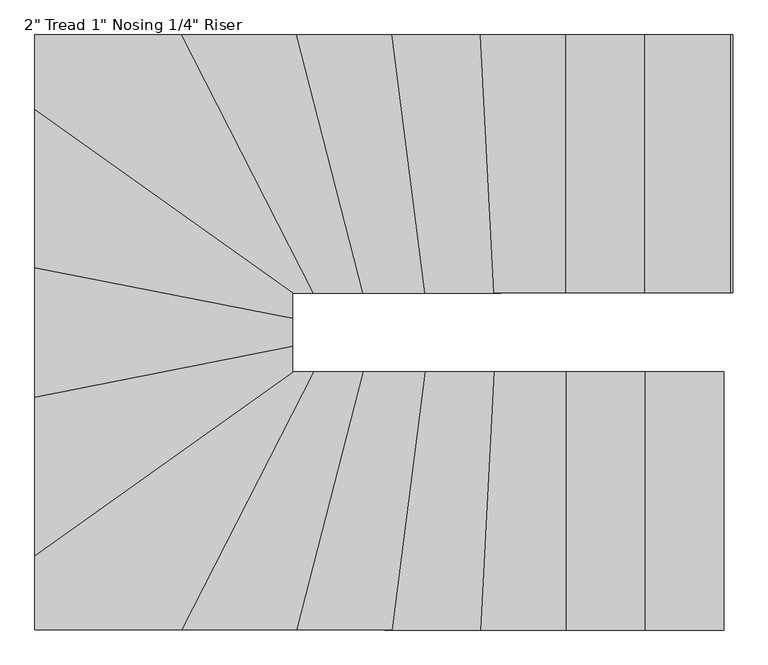
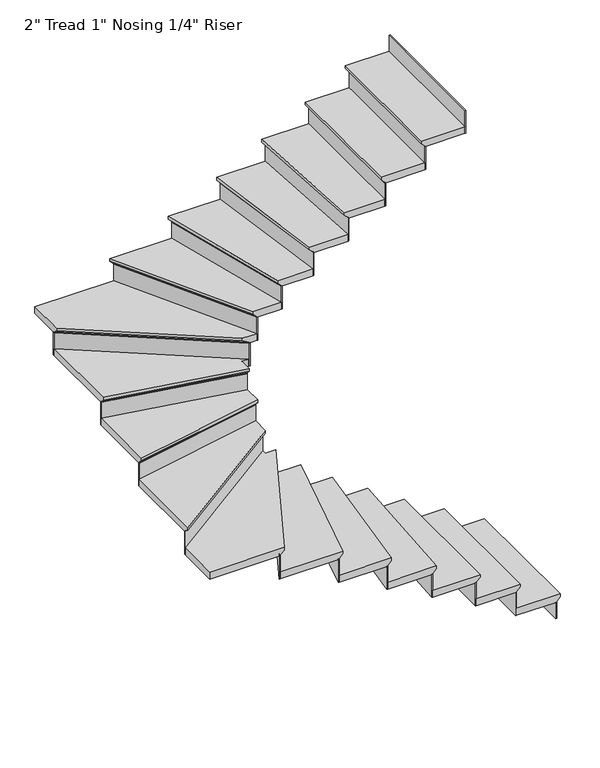
"""IFC4 building model written with IfcOpenShell, lengths in millimetres: stair flight geometry."""

from ifc_helpers import new_model, si_unit, origin, place, context, project, spatial, faceted_brep, source, transform, mapped, element, save


def stair_flight_5a9f065b(model_context):
    return source(origin(), model_context, "Body", "Brep", [
        faceted_brep([(-1761.7449167, -345.7070853, 150.2833333), (-1761.7449167, -345.7070853, 169.3333333), (-1761.7449167, -1260.1070853, 169.3333333), (-1761.7449167, -1260.1070853, 150.2833333), (-1787.1449167, -345.7070853, 124.8833333), (-1787.1449167, -1260.1070853, 124.8833333), (-2066.5449167, -345.7070853, 169.3333333), (-2066.5449167, -1260.1070853, 169.3333333), (-1787.1449167, -1260.1070853, 118.5333333), (-2066.5449167, -1260.1070853, 118.5333333), (-2066.5449167, -345.7070853, 118.5333333), (-1787.1449167, -345.7070853, 118.5333333)], [[[0, 1, 2, 3]], [[4, 0, 3, 5]], [[2, 1, 6, 7]], [[8, 9, 10, 11]], [[2, 7, 9, 8, 5, 3]], [[8, 11, 4, 5]], [[6, 1, 0, 4, 11, 10]], [[7, 6, 10, 9]]]),
        faceted_brep([(-1787.1449167, -345.7070853, 118.5333333), (-1787.1449167, -345.7070853, 0.0), (-1793.4949167, -345.7070853, 0.0), (-1793.4949167, -345.7070853, 118.5333333), (-1787.1449167, -1260.1070853, 118.5333333), (-1793.4949167, -1260.1070853, 118.5333333), (-1793.4949167, -1260.1070853, 0.0), (-1787.1449167, -1260.1070853, 0.0)], [[[0, 1, 2, 3]], [[4, 5, 6, 7]], [[1, 0, 4, 7]], [[2, 1, 7, 6]], [[3, 2, 6, 5]], [[0, 3, 5, 4]]]),
        faceted_brep([(-2066.5449167, -345.7070853, 287.8666667), (-2066.5449167, -345.7070853, 118.5333333), (-2072.8949167, -345.7070853, 118.5333333), (-2072.8949167, -345.7070853, 287.8666667), (-2066.5449167, -1260.1070853, 287.8666667), (-2072.8949167, -1260.1070853, 287.8666667), (-2072.8949167, -1260.1070853, 118.5333333), (-2066.5449167, -1260.1070853, 118.5333333)], [[[0, 1, 2, 3]], [[4, 5, 6, 7]], [[1, 0, 4, 7]], [[2, 1, 7, 6]], [[3, 2, 6, 5]], [[0, 3, 5, 4]]]),
        faceted_brep([(-2041.1449167, -1260.1070853, 338.6666667), (-2041.1449167, -345.7070853, 338.6666667), (-2345.9449167, -345.7070853, 338.6666667), (-2345.9449167, -1260.1070853, 338.6666667), (-2066.5449167, -1260.1070853, 287.8666667), (-2345.9449167, -1260.1070853, 287.8666667), (-2345.9449167, -345.7070853, 287.8666667), (-2066.5449167, -345.7070853, 287.8666667), (-2066.5449167, -1260.1070853, 294.2166667), (-2041.1449167, -1260.1070853, 319.6166667), (-2066.5449167, -345.7070853, 294.2166667), (-2041.1449167, -345.7070853, 319.6166667)], [[[0, 1, 2, 3]], [[4, 5, 6, 7]], [[0, 3, 5, 4, 8, 9]], [[4, 7, 10, 8]], [[2, 1, 11, 10, 7, 6]], [[3, 2, 6, 5]], [[11, 1, 0, 9]], [[10, 11, 9, 8]]]),
        faceted_brep([(-2345.9449167, -345.7070853, 457.2), (-2345.9449167, -345.7070853, 287.8666667), (-2352.2949167, -345.7070853, 287.8666667), (-2352.2949167, -345.7070853, 457.2), (-2345.9449167, -1260.1070853, 457.2), (-2352.2949167, -1260.1070853, 457.2), (-2352.2949167, -1260.1070853, 287.8666667), (-2345.9449167, -1260.1070853, 287.8666667)], [[[0, 1, 2, 3]], [[4, 5, 6, 7]], [[1, 0, 4, 7]], [[2, 1, 7, 6]], [[3, 2, 6, 5]], [[0, 3, 5, 4]]]),
        faceted_brep([(-2320.5449167, -1260.1070853, 508.0), (-2320.5449167, -345.7070853, 508.0), (-2601.6120781, -345.7070853, 508.0), (-2649.1463485, -1260.1070853, 508.0), (-2345.9449167, -1260.1070853, 457.2), (-2649.1463485, -1260.1070853, 457.2), (-2601.6120781, -345.7070853, 457.2), (-2345.9449167, -345.7070853, 457.2), (-2345.9449167, -1260.1070853, 463.55), (-2320.5449167, -1260.1070853, 488.95), (-2345.9449167, -345.7070853, 463.55), (-2320.5449167, -345.7070853, 488.95)], [[[0, 1, 2, 3]], [[4, 5, 6, 7]], [[0, 3, 5, 4, 8, 9]], [[4, 7, 10, 8]], [[2, 1, 11, 10, 7, 6]], [[3, 2, 6, 5]], [[11, 1, 0, 9]], [[10, 11, 9, 8]]]),
        faceted_brep([(-2601.6120781, -345.7070853, 626.5333333), (-2601.6120781, -345.7070853, 457.2), (-2607.9706523, -345.7070853, 457.2), (-2607.9706523, -345.7070853, 626.5333333), (-2649.1463485, -1260.1070853, 626.5333333), (-2655.5049227, -1260.1070853, 626.5333333), (-2655.5049227, -1260.1070853, 457.2), (-2649.1463485, -1260.1070853, 457.2)], [[[0, 1, 2, 3]], [[4, 5, 6, 7]], [[1, 0, 4, 7]], [[2, 1, 7, 6]], [[3, 2, 6, 5]], [[0, 3, 5, 4]]]),
        faceted_brep([(-2623.7120519, -1260.1070853, 677.3333333), (-2576.1777815, -345.7070853, 677.3333333), (-2845.778778, -345.7070853, 677.3333333), (-2964.1348296, -1260.1070853, 677.3333333), (-2649.1463485, -1260.1070853, 626.5333333), (-2964.1348296, -1260.1070853, 626.5333333), (-2845.778778, -345.7070853, 626.5333333), (-2601.6120781, -345.7070853, 626.5333333), (-2649.1463485, -1260.1070853, 632.8833333), (-2623.7120519, -1260.1070853, 658.2833333), (-2601.6120781, -345.7070853, 632.8833333), (-2576.1777815, -345.7070853, 658.2833333)], [[[0, 1, 2, 3]], [[4, 5, 6, 7]], [[0, 3, 5, 4, 8, 9]], [[4, 7, 10, 8]], [[2, 1, 11, 10, 7, 6]], [[3, 2, 6, 5]], [[11, 1, 0, 9]], [[10, 11, 9, 8]]]),
        faceted_brep([(-2845.778778, -345.7070853, 795.8666667), (-2845.778778, -345.7070853, 626.5333333), (-2852.1817497, -345.7070853, 626.5333333), (-2852.1817497, -345.7070853, 795.8666667), (-2964.1348296, -1260.1070853, 795.8666667), (-2970.5378014, -1260.1070853, 795.8666667), (-2970.5378014, -1260.1070853, 626.5333333), (-2964.1348296, -1260.1070853, 626.5333333)], [[[0, 1, 2, 3]], [[4, 5, 6, 7]], [[1, 0, 4, 7]], [[2, 1, 7, 6]], [[3, 2, 6, 5]], [[0, 3, 5, 4]]]),
        faceted_brep([(-2938.5229425, -1260.1070853, 846.6666667), (-2820.1668908, -345.7070853, 846.6666667), (-3067.4060004, -345.7070853, 846.6666667), (-3302.5364478, -1260.1070853, 846.6666667), (-2964.1348296, -1260.1070853, 795.8666667), (-3302.5364478, -1260.1070853, 795.8666667), (-3067.4060004, -345.7070853, 795.8666667), (-2845.778778, -345.7070853, 795.8666667), (-2964.1348296, -1260.1070853, 802.2166667), (-2938.5229425, -1260.1070853, 827.6166667), (-2845.778778, -345.7070853, 802.2166667), (-2820.1668908, -345.7070853, 827.6166667)], [[[0, 1, 2, 3]], [[4, 5, 6, 7]], [[0, 3, 5, 4, 8, 9]], [[4, 7, 10, 8]], [[2, 1, 11, 10, 7, 6]], [[3, 2, 6, 5]], [[11, 1, 0, 9]], [[10, 11, 9, 8]]]),
        faceted_brep([(-3067.4060004, -345.7070853, 965.2), (-3067.4060004, -345.7070853, 795.8666667), (-3073.9625773, -345.7070853, 795.8666667), (-3073.9625773, -345.7070853, 965.2), (-3302.5364478, -1260.1070853, 965.2), (-3309.0930247, -1260.1070853, 965.2), (-3309.0930247, -1260.1070853, 795.8666667), (-3302.5364478, -1260.1070853, 795.8666667)], [[[0, 1, 2, 3]], [[4, 5, 6, 7]], [[1, 0, 4, 7]], [[2, 1, 7, 6]], [[3, 2, 6, 5]], [[0, 3, 5, 4]]]),
        faceted_brep([(-3276.3101404, -1260.1070853, 1016.0), (-3041.179693, -345.7070853, 1016.0), (-3243.7526365, -345.7070853, 1016.0), (-3712.5772578, -1260.1070853, 1016.0), (-3302.5364478, -1260.1070853, 965.2), (-3712.5772578, -1260.1070853, 965.2), (-3243.7526365, -345.7070853, 965.2), (-3067.4060004, -345.7070853, 965.2), (-3302.5364478, -1260.1070853, 971.55), (-3276.3101404, -1260.1070853, 996.95), (-3067.4060004, -345.7070853, 971.55), (-3041.179693, -345.7070853, 996.95)], [[[0, 1, 2, 3]], [[4, 5, 6, 7]], [[0, 3, 5, 4, 8, 9]], [[4, 7, 10, 8]], [[2, 1, 11, 10, 7, 6]], [[3, 2, 6, 5]], [[11, 1, 0, 9]], [[10, 11, 9, 8]]]),
        faceted_brep([(-3243.7526365, -345.7070853, 1134.5333333), (-3243.7526365, -345.7070853, 965.2), (-3250.8886197, -345.7070853, 965.2), (-3250.8886197, -345.7070853, 1134.5333333), (-3712.5772578, -1260.1070853, 1134.5333333), (-3719.713241, -1260.1070853, 1134.5333333), (-3719.713241, -1260.1070853, 965.2), (-3712.5772578, -1260.1070853, 965.2)], [[[0, 1, 2, 3]], [[4, 5, 6, 7]], [[1, 0, 4, 7]], [[2, 1, 7, 6]], [[3, 2, 6, 5]], [[0, 3, 5, 4]]]),
        faceted_brep([(-4203.8766085, -966.4259516, 1185.3333333), (-4203.8766085, -1260.1070853, 1185.3333333), (-3684.0333253, -1260.1070853, 1185.3333333), (-3215.208704, -345.7070853, 1185.3333333), (-3289.4766085, -345.7070853, 1185.3333333), (-3289.4766085, -316.1520025, 1185.3333333), (-4203.8766085, -1260.1070853, 1134.5333333), (-4203.8766085, -966.4259516, 1134.5333333), (-3289.4766085, -316.1520025, 1134.5333333), (-3289.4766085, -345.7070853, 1134.5333333), (-3243.7526365, -345.7070853, 1134.5333333), (-3712.5772578, -1260.1070853, 1134.5333333), (-3712.5772578, -1260.1070853, 1140.8833333), (-3684.0333253, -1260.1070853, 1166.2833333), (-3243.7526365, -345.7070853, 1140.8833333), (-3215.208704, -345.7070853, 1166.2833333)], [[[0, 1, 2, 3, 4, 5]], [[6, 7, 8, 9, 10, 11]], [[1, 0, 7, 6]], [[2, 1, 6, 11, 12, 13]], [[11, 10, 14, 12]], [[4, 3, 15, 14, 10, 9]], [[5, 4, 9, 8]], [[0, 5, 8, 7]], [[15, 3, 2, 13]], [[14, 15, 13, 12]]]),
        faceted_brep([(-3289.4766085, -316.1520025, 1303.8666667), (-3289.4766085, -316.1520025, 1134.5333333), (-3289.4766085, -308.3600277, 1134.5333333), (-3289.4766085, -308.3600277, 1303.8666667), (-4203.8766085, -966.4259516, 1303.8666667), (-4203.8766085, -958.6339768, 1303.8666667), (-4203.8766085, -958.6339768, 1134.5333333), (-4203.8766085, -966.4259516, 1134.5333333)], [[[0, 1, 2, 3]], [[4, 5, 6, 7]], [[1, 0, 4, 7]], [[2, 1, 7, 6]], [[3, 2, 6, 5]], [[0, 3, 5, 4]]]),
        faceted_brep([(-4203.8766085, -997.5938508, 1354.6666667), (-3289.4766085, -347.3199017, 1354.6666667), (-3289.4766085, -229.6979154, 1354.6666667), (-4203.8766085, -409.9387717, 1354.6666667), (-4203.8766085, -966.4259516, 1303.8666667), (-4203.8766085, -409.9387717, 1303.8666667), (-3289.4766085, -229.6979154, 1303.8666667), (-3289.4766085, -316.1520025, 1303.8666667), (-4203.8766085, -966.4259516, 1310.2166667), (-4203.8766085, -997.5938508, 1335.6166667), (-3289.4766085, -316.1520025, 1310.2166667), (-3289.4766085, -347.3199017, 1335.6166667)], [[[0, 1, 2, 3]], [[4, 5, 6, 7]], [[0, 3, 5, 4, 8, 9]], [[4, 7, 10, 8]], [[2, 1, 11, 10, 7, 6]], [[3, 2, 6, 5]], [[11, 1, 0, 9]], [[10, 11, 9, 8]]]),
        faceted_brep([(-3289.4766085, -229.6979154, 1473.2), (-3289.4766085, -229.6979154, 1303.8666667), (-3289.4766085, -223.22573, 1303.8666667), (-3289.4766085, -223.22573, 1473.2), (-4203.8766085, -409.9387717, 1473.2), (-4203.8766085, -403.4665863, 1473.2), (-4203.8766085, -403.4665863, 1303.8666667), (-4203.8766085, -409.9387717, 1303.8666667)], [[[0, 1, 2, 3]], [[4, 5, 6, 7]], [[1, 0, 4, 7]], [[2, 1, 7, 6]], [[3, 2, 6, 5]], [[0, 3, 5, 4]]]),
        faceted_brep([(-4203.8766085, -435.8275135, 1524.0), (-3289.4766085, -255.5866572, 1524.0), (-3289.4766085, -130.5387717, 1524.0), (-4203.8766085, 49.7020846, 1524.0), (-4203.8766085, -409.9387717, 1473.2), (-4203.8766085, 49.7020846, 1473.2), (-3289.4766085, -130.5387717, 1473.2), (-3289.4766085, -229.6979154, 1473.2), (-4203.8766085, -409.9387717, 1479.55), (-4203.8766085, -435.8275135, 1504.95), (-3289.4766085, -229.6979154, 1479.55), (-3289.4766085, -255.5866572, 1504.95)], [[[0, 1, 2, 3]], [[4, 5, 6, 7]], [[0, 3, 5, 4, 8, 9]], [[4, 7, 10, 8]], [[2, 1, 11, 10, 7, 6]], [[3, 2, 6, 5]], [[11, 1, 0, 9]], [[10, 11, 9, 8]]]),
        faceted_brep([(-3289.4766085, -130.5387717, 1642.5333333), (-3289.4766085, -130.5387717, 1473.2), (-3289.4766085, -124.0665863, 1473.2), (-3289.4766085, -124.0665863, 1642.5333333), (-4203.8766085, 49.7020846, 1642.5333333), (-4203.8766085, 56.17427, 1642.5333333), (-4203.8766085, 56.17427, 1473.2), (-4203.8766085, 49.7020846, 1473.2)], [[[0, 1, 2, 3]], [[4, 5, 6, 7]], [[1, 0, 4, 7]], [[2, 1, 7, 6]], [[3, 2, 6, 5]], [[0, 3, 5, 4]]]),
        faceted_brep([(-4203.8766085, 23.8133428, 1693.3333333), (-3289.4766085, -156.4275135, 1693.3333333), (-3289.4766085, -66.3070853, 1693.3333333), (-3243.381134, -66.3070853, 1693.3333333), (-4203.8766085, 616.7475793, 1693.3333333), (-4203.8766085, 49.7020846, 1642.5333333), (-4203.8766085, 616.7475793, 1642.5333333), (-3243.381134, -66.3070853, 1642.5333333), (-3289.4766085, -66.3070853, 1642.5333333), (-3289.4766085, -130.5387717, 1642.5333333), (-4203.8766085, 49.7020846, 1648.8833333), (-4203.8766085, 23.8133428, 1674.2833333), (-3289.4766085, -130.5387717, 1648.8833333), (-3289.4766085, -156.4275135, 1674.2833333)], [[[0, 1, 2, 3, 4]], [[5, 6, 7, 8, 9]], [[0, 4, 6, 5, 10, 11]], [[5, 9, 12, 10]], [[2, 1, 13, 12, 9, 8]], [[3, 2, 8, 7]], [[4, 3, 7, 6]], [[13, 1, 0, 11]], [[12, 13, 11, 10]]]),
        faceted_brep([(-3243.381134, -66.3070853, 1811.8666667), (-3243.381134, -66.3070853, 1642.5333333), (-3232.4242415, -66.3070853, 1642.5333333), (-3232.4242415, -66.3070853, 1811.8666667), (-4203.8766085, 616.7475793, 1811.8666667), (-4203.8766085, 624.5395541, 1811.8666667), (-4203.8766085, 624.5395541, 1642.5333333), (-4203.8766085, 616.7475793, 1642.5333333)], [[[0, 1, 2, 3]], [[4, 5, 6, 7]], [[1, 0, 4, 7]], [[2, 1, 7, 6]], [[3, 2, 6, 5]], [[0, 3, 5, 4]]]),
        faceted_brep([(-3655.4893928, 848.0929147, 1862.6666667), (-4203.8766085, 848.0929147, 1862.6666667), (-4203.8766085, 585.5796802, 1862.6666667), (-3287.208704, -66.3070853, 1862.6666667), (-3186.6647715, -66.3070853, 1862.6666667), (-4203.8766085, 848.0929147, 1811.8666667), (-3655.4893928, 848.0929147, 1811.8666667), (-3186.6647715, -66.3070853, 1811.8666667), (-3243.381134, -66.3070853, 1811.8666667), (-4203.8766085, 616.7475793, 1811.8666667), (-4203.8766085, 616.7475793, 1818.2166667), (-4203.8766085, 585.5796802, 1843.6166667), (-3243.381134, -66.3070853, 1818.2166667), (-3287.208704, -66.3070853, 1843.6166667)], [[[0, 1, 2, 3, 4]], [[5, 6, 7, 8, 9]], [[1, 0, 6, 5]], [[2, 1, 5, 9, 10, 11]], [[9, 8, 12, 10]], [[4, 3, 13, 12, 8, 7]], [[0, 4, 7, 6]], [[13, 3, 2, 11]], [[12, 13, 11, 10]]]),
        faceted_brep([(-3186.6647715, -66.3070853, 1981.2), (-3186.6647715, -66.3070853, 1811.8666667), (-3179.5287883, -66.3070853, 1811.8666667), (-3179.5287883, -66.3070853, 1981.2), (-3655.4893928, 848.0929147, 1981.2), (-3648.3534096, 848.0929147, 1981.2), (-3648.3534096, 848.0929147, 1811.8666667), (-3655.4893928, 848.0929147, 1811.8666667)], [[[0, 1, 2, 3]], [[4, 5, 6, 7]], [[1, 0, 4, 7]], [[2, 1, 7, 6]], [[3, 2, 6, 5]], [[0, 3, 5, 4]]]),
        faceted_brep([(-3684.0333253, 848.0929147, 2032.0), (-3215.208704, -66.3070853, 2032.0), (-3014.9533855, -66.3070853, 2032.0), (-3250.0838329, 848.0929147, 2032.0), (-3655.4893928, 848.0929147, 1981.2), (-3250.0838329, 848.0929147, 1981.2), (-3014.9533855, -66.3070853, 1981.2), (-3186.6647715, -66.3070853, 1981.2), (-3655.4893928, 848.0929147, 1987.55), (-3684.0333253, 848.0929147, 2012.95), (-3186.6647715, -66.3070853, 1987.55), (-3215.208704, -66.3070853, 2012.95)], [[[0, 1, 2, 3]], [[4, 5, 6, 7]], [[0, 3, 5, 4, 8, 9]], [[4, 7, 10, 8]], [[2, 1, 11, 10, 7, 6]], [[3, 2, 6, 5]], [[11, 1, 0, 9]], [[10, 11, 9, 8]]]),
        faceted_brep([(-3014.9533855, -66.3070853, 2150.5333333), (-3014.9533855, -66.3070853, 1981.2), (-3008.3968086, -66.3070853, 1981.2), (-3008.3968086, -66.3070853, 2150.5333333), (-3250.0838329, 848.0929147, 2150.5333333), (-3243.5272561, 848.0929147, 2150.5333333), (-3243.5272561, 848.0929147, 1981.2), (-3250.0838329, 848.0929147, 1981.2)], [[[0, 1, 2, 3]], [[4, 5, 6, 7]], [[1, 0, 4, 7]], [[2, 1, 7, 6]], [[3, 2, 6, 5]], [[0, 3, 5, 4]]]),
        faceted_brep([(-3276.3101404, 848.0929147, 2201.3333333), (-3041.179693, -66.3070853, 2201.3333333), (-2794.5550037, -66.3070853, 2201.3333333), (-2912.9110554, 848.0929147, 2201.3333333), (-3250.0838329, 848.0929147, 2150.5333333), (-2912.9110554, 848.0929147, 2150.5333333), (-2794.5550037, -66.3070853, 2150.5333333), (-3014.9533855, -66.3070853, 2150.5333333), (-3250.0838329, 848.0929147, 2156.8833333), (-3276.3101404, 848.0929147, 2182.2833333), (-3014.9533855, -66.3070853, 2156.8833333), (-3041.179693, -66.3070853, 2182.2833333)], [[[0, 1, 2, 3]], [[4, 5, 6, 7]], [[0, 3, 5, 4, 8, 9]], [[4, 7, 10, 8]], [[2, 1, 11, 10, 7, 6]], [[3, 2, 6, 5]], [[11, 1, 0, 9]], [[10, 11, 9, 8]]]),
        faceted_brep([(-2794.5550037, -66.3070853, 2319.8666667), (-2794.5550037, -66.3070853, 2150.5333333), (-2788.152032, -66.3070853, 2150.5333333), (-2788.152032, -66.3070853, 2319.8666667), (-2912.9110554, 848.0929147, 2319.8666667), (-2906.5080836, 848.0929147, 2319.8666667), (-2906.5080836, 848.0929147, 2150.5333333), (-2912.9110554, 848.0929147, 2150.5333333)], [[[0, 1, 2, 3]], [[4, 5, 6, 7]], [[1, 0, 4, 7]], [[2, 1, 7, 6]], [[3, 2, 6, 5]], [[0, 3, 5, 4]]]),
        faceted_brep([(-2938.5229425, 848.0929147, 2370.6666667), (-2820.1668908, -66.3070853, 2370.6666667), (-2550.7434848, -66.3070853, 2370.6666667), (-2598.2777552, 848.0929147, 2370.6666667), (-2912.9110554, 848.0929147, 2319.8666667), (-2598.2777552, 848.0929147, 2319.8666667), (-2550.7434848, -66.3070853, 2319.8666667), (-2794.5550037, -66.3070853, 2319.8666667), (-2912.9110554, 848.0929147, 2326.2166667), (-2938.5229425, 848.0929147, 2351.6166667), (-2794.5550037, -66.3070853, 2326.2166667), (-2820.1668908, -66.3070853, 2351.6166667)], [[[0, 1, 2, 3]], [[4, 5, 6, 7]], [[0, 3, 5, 4, 8, 9]], [[4, 7, 10, 8]], [[2, 1, 11, 10, 7, 6]], [[3, 2, 6, 5]], [[11, 1, 0, 9]], [[10, 11, 9, 8]]]),
        faceted_brep([(-2550.7434848, -66.3070853, 2489.2), (-2550.7434848, -66.3070853, 2319.8666667), (-2544.3849106, -66.3070853, 2319.8666667), (-2544.3849106, -66.3070853, 2489.2), (-2598.2777552, 848.0929147, 2489.2), (-2591.9191811, 848.0929147, 2489.2), (-2591.9191811, 848.0929147, 2319.8666667), (-2598.2777552, 848.0929147, 2319.8666667)], [[[0, 1, 2, 3]], [[4, 5, 6, 7]], [[1, 0, 4, 7]], [[2, 1, 7, 6]], [[3, 2, 6, 5]], [[0, 3, 5, 4]]]),
        faceted_brep([(-2623.7120519, 848.0929147, 2540.0), (-2576.1777815, -66.3070853, 2540.0), (-2295.1449167, -66.3070853, 2540.0), (-2295.1449167, 848.0929147, 2540.0), (-2598.2777552, 848.0929147, 2489.2), (-2295.1449167, 848.0929147, 2489.2), (-2295.1449167, -66.3070853, 2489.2), (-2550.7434848, -66.3070853, 2489.2), (-2598.2777552, 848.0929147, 2495.55), (-2623.7120519, 848.0929147, 2520.95), (-2550.7434848, -66.3070853, 2495.55), (-2576.1777815, -66.3070853, 2520.95)], [[[0, 1, 2, 3]], [[4, 5, 6, 7]], [[0, 3, 5, 4, 8, 9]], [[4, 7, 10, 8]], [[2, 1, 11, 10, 7, 6]], [[3, 2, 6, 5]], [[11, 1, 0, 9]], [[10, 11, 9, 8]]]),
        faceted_brep([(-2295.1449167, -66.3070853, 2658.5333333), (-2295.1449167, -66.3070853, 2489.2), (-2288.7949167, -66.3070853, 2489.2), (-2288.7949167, -66.3070853, 2658.5333333), (-2295.1449167, 848.0929147, 2658.5333333), (-2288.7949167, 848.0929147, 2658.5333333), (-2288.7949167, 848.0929147, 2489.2), (-2295.1449167, 848.0929147, 2489.2)], [[[0, 1, 2, 3]], [[4, 5, 6, 7]], [[1, 0, 4, 7]], [[2, 1, 7, 6]], [[3, 2, 6, 5]], [[0, 3, 5, 4]]]),
        faceted_brep([(-2320.5449167, 848.0929147, 2709.3333333), (-2320.5449167, -66.3070853, 2709.3333333), (-2015.7449167, -66.3070853, 2709.3333333), (-2015.7449167, 848.0929147, 2709.3333333), (-2295.1449167, 848.0929147, 2658.5333333), (-2015.7449167, 848.0929147, 2658.5333333), (-2015.7449167, -66.3070853, 2658.5333333), (-2295.1449167, -66.3070853, 2658.5333333), (-2295.1449167, 848.0929147, 2664.8833333), (-2320.5449167, 848.0929147, 2690.2833333), (-2295.1449167, -66.3070853, 2664.8833333), (-2320.5449167, -66.3070853, 2690.2833333)], [[[0, 1, 2, 3]], [[4, 5, 6, 7]], [[0, 3, 5, 4, 8, 9]], [[4, 7, 10, 8]], [[2, 1, 11, 10, 7, 6]], [[3, 2, 6, 5]], [[11, 1, 0, 9]], [[10, 11, 9, 8]]]),
        faceted_brep([(-2015.7449167, -66.3070853, 2827.8666667), (-2015.7449167, -66.3070853, 2658.5333333), (-2009.3949167, -66.3070853, 2658.5333333), (-2009.3949167, -66.3070853, 2827.8666667), (-2015.7449167, 848.0929147, 2827.8666667), (-2009.3949167, 848.0929147, 2827.8666667), (-2009.3949167, 848.0929147, 2658.5333333), (-2015.7449167, 848.0929147, 2658.5333333)], [[[0, 1, 2, 3]], [[4, 5, 6, 7]], [[1, 0, 4, 7]], [[2, 1, 7, 6]], [[3, 2, 6, 5]], [[0, 3, 5, 4]]]),
        faceted_brep([(-1736.3449167, -66.3070853, 2997.2), (-1736.3449167, -66.3070853, 2827.8666667), (-1729.9949167, -66.3070853, 2827.8666667), (-1729.9949167, -66.3070853, 2997.2), (-1736.3449167, 848.0929147, 2997.2), (-1729.9949167, 848.0929147, 2997.2), (-1729.9949167, 848.0929147, 2827.8666667), (-1736.3449167, 848.0929147, 2827.8666667)], [[[0, 1, 2, 3]], [[4, 5, 6, 7]], [[1, 0, 4, 7]], [[2, 1, 7, 6]], [[3, 2, 6, 5]], [[0, 3, 5, 4]]]),
        faceted_brep([(-2041.1449167, 848.0929147, 2878.6666667), (-2041.1449167, -66.3070853, 2878.6666667), (-1736.3449167, -66.3070853, 2878.6666667), (-1736.3449167, 848.0929147, 2878.6666667), (-2015.7449167, 848.0929147, 2827.8666667), (-1736.3449167, 848.0929147, 2827.8666667), (-1736.3449167, -66.3070853, 2827.8666667), (-2015.7449167, -66.3070853, 2827.8666667), (-2015.7449167, 848.0929147, 2834.2166667), (-2041.1449167, 848.0929147, 2859.6166667), (-2015.7449167, -66.3070853, 2834.2166667), (-2041.1449167, -66.3070853, 2859.6166667)], [[[0, 1, 2, 3]], [[4, 5, 6, 7]], [[0, 3, 5, 4, 8, 9]], [[4, 7, 10, 8]], [[2, 1, 11, 10, 7, 6]], [[3, 2, 6, 5]], [[11, 1, 0, 9]], [[10, 11, 9, 8]]]),
    ])


if __name__ == "__main__":
    model = new_model("IFC4")
    model_context = context("Model", 3, world=origin())
    ifc_project = project(units=[si_unit("LENGTHUNIT", "METRE", prefix="MILLI")], contexts=[model_context])
    site = spatial("IfcSite", under=ifc_project)
    building = spatial("IfcBuilding", under=site)
    placement = place(None, origin())
    stair_flight_shape = stair_flight_5a9f065b(model_context)
    element("IfcStairFlight", 1, ObjectType="2\" Tread 1\" Nosing 1/4\" Riser", at=placement, inside=building, context=model_context, shape_type="MappedRepresentation", body=[
        mapped(stair_flight_shape, transform((0.0, 0.0, 0.0), x_axis=(1.0, 0.0, 0.0), y_axis=(0.0, 1.0, 0.0), z_axis=(0.0, 0.0, 1.0))),
    ])
    save(model, "model.ifc")
